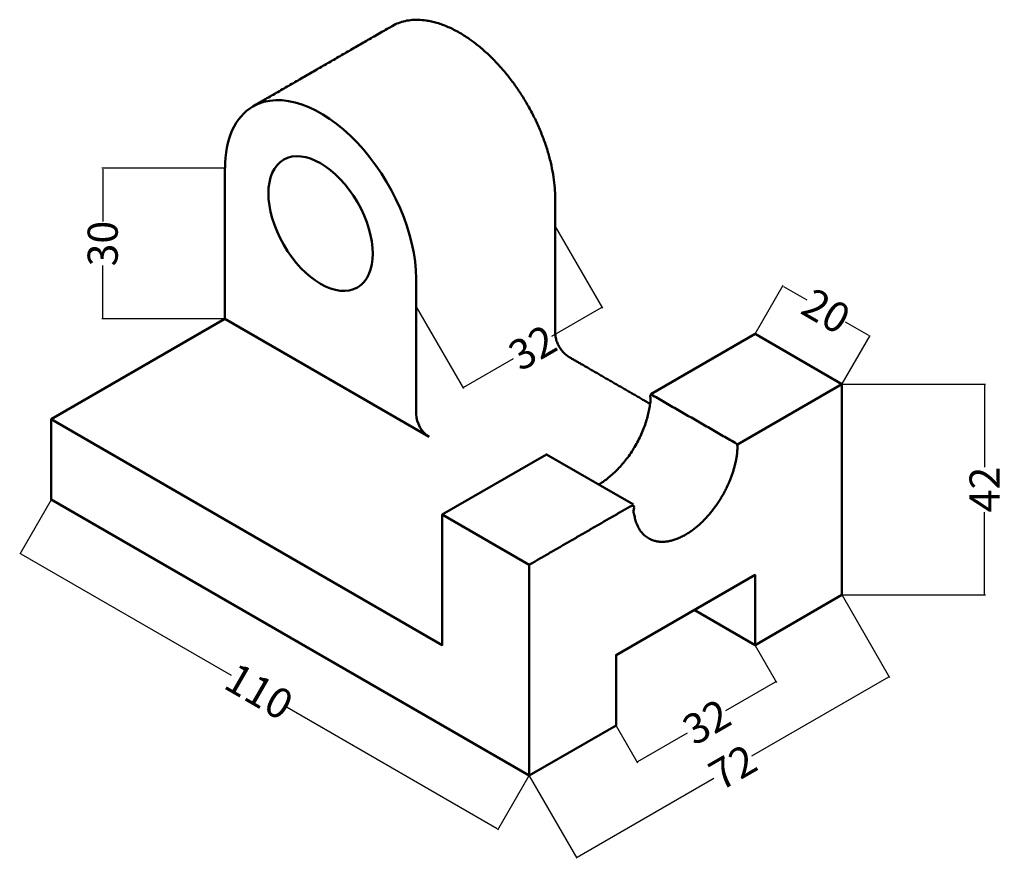
# Model space of a CAD drawing. Units: millimetres. Extents: x -6 to 190, y -9 to 158.
import ezdxf

# ---------------------------------------------------------------- set-up
doc = ezdxf.new("R2010")
doc.units = ezdxf.units.MM
doc.header["$MEASUREMENT"] = 0
doc.layers.add('M-DIMS', color=2, linetype='Continuous', lineweight=25)
doc.layers.add('M-OUTL', color=7, linetype='Continuous', lineweight=50)
doc.styles.get("Standard").update_dxf_attribs({"font": 'arial.ttf'})
doc.dimstyles.get("Standard").update_dxf_attribs({"dimtxt": 6, "dimasz": 0.18, "dimexe": 0.18, "dimexo": 0.0625, "dimgap": 0.09, "dimtad": 0, "dimtoh": 1, "dimdec": 0, "dimzin": 0, "dimdsep": 46, "dimtxsty": 'Standard', "dimcen": 0.09, "dimadec": 0, "dimazin": 0, "dimtfac": 1, "dimtdec": 0, "dimtofl": 0, "dimtmove": 0, "dimatfit": 3, "dimfxl": 1, "dimtolj": 1, "dimtzin": 0, "dimarcsym": 0})

# ---------------------------------------------------------------- blocks, each defined once
blk = doc.blocks.new('*D1')
at = {"layer": 'Defpoints', "color": 0, "transparency": 16777216}
for p in [(157.45, 85.07), (157.45, 43.07), (185.88, 43.07)]:
    blk.add_point(p, dxfattribs=at)
at = {"layer": 'M-DIMS', "color": 0, "lineweight": -2, "transparency": 16777216}
for p, q in [((157.51, 85.07), (186.06, 85.07)), ((185.88, 84.89), (185.88, 68.55)), ((185.88, 43.25), (185.88, 59.59)), ((157.51, 43.07), (186.06, 43.07))]:
    blk.add_line(p, q, dxfattribs=at)
at = {"layer": 'M-DIMS', "color": 0, "transparency": 16777216}
for points in [[(185.85, 84.89), (185.91, 84.89), (185.88, 85.07)], [(185.85, 43.25), (185.91, 43.25), (185.88, 43.07)]]:
    blk.add_solid(points, dxfattribs=at)
at = {"layer": 'M-DIMS', "color": 0, "transparency": 16777216, "insert": (185.88, 64.07), "char_height": 6, "attachment_point": 5, "rotation": 90}
blk.add_mtext('\\A1;42', dxfattribs=at)
blk = doc.blocks.new('*D2')
at = {"layer": 'Defpoints', "color": 0, "transparency": 16777216}
for p in [(-0.17, 62.07), (95.1, 7.07), (88.91, -3.65)]:
    blk.add_point(p, dxfattribs=at)
at = {"layer": 'M-DIMS', "color": 0, "lineweight": -2, "transparency": 16777216}
for p, q in [((-0.2, 62.02), (-6.45, 51.2)), ((-6.2, 51.26), (35.71, 27.07)), ((88.75, -3.56), (46.84, 20.64)), ((95.06, 7.02), (88.82, -3.8))]:
    blk.add_line(p, q, dxfattribs=at)
at = {"layer": 'M-DIMS', "color": 0, "transparency": 16777216}
for points in [[(-6.18, 51.29), (-6.21, 51.24), (-6.36, 51.35)], [(88.77, -3.53), (88.74, -3.58), (88.91, -3.65)]]:
    blk.add_solid(points, dxfattribs=at)
at = {"layer": 'M-DIMS', "color": 0, "transparency": 16777216, "insert": (41.28, 23.85), "char_height": 6, "attachment_point": 5, "rotation": 330}
blk.add_mtext('\\A1;110', dxfattribs=at)
blk = doc.blocks.new('*D3')
at = {"layer": 'Defpoints', "color": 0, "transparency": 16777216}
for p in [(157.45, 43.07), (166.87, 26.75), (95.1, 7.07)]:
    blk.add_point(p, dxfattribs=at)
at = {"layer": 'M-DIMS', "color": 0, "lineweight": -2, "transparency": 16777216}
for p, q in [((157.48, 43.02), (166.96, 26.6)), ((166.71, 26.66), (139.45, 10.92)), ((95.13, 7.02), (104.61, -9.4)), ((104.67, -9.16), (131.94, 6.59))]:
    blk.add_line(p, q, dxfattribs=at)
at = {"layer": 'M-DIMS', "color": 0, "transparency": 16777216}
for points in [[(166.7, 26.69), (166.73, 26.64), (166.87, 26.75)], [(104.66, -9.13), (104.69, -9.18), (104.52, -9.25)]]:
    blk.add_solid(points, dxfattribs=at)
at = {"layer": 'M-DIMS', "color": 0, "transparency": 16777216, "insert": (135.69, 8.75), "char_height": 6, "attachment_point": 5, "rotation": 30}
blk.add_mtext('\\A1;72', dxfattribs=at)
blk = doc.blocks.new('*D4')
at = {"layer": 'Defpoints', "color": 0, "transparency": 16777216}
for p in [(140.13, 33.07), (144.33, 25.79), (112.42, 17.07)]:
    blk.add_point(p, dxfattribs=at)
at = {"layer": 'M-DIMS', "color": 0, "lineweight": -2, "transparency": 16777216}
for p, q in [((140.16, 33.02), (144.42, 25.64)), ((144.17, 25.7), (134.24, 19.97)), ((112.45, 17.02), (116.71, 9.64)), ((116.77, 9.88), (126.7, 15.62))]:
    blk.add_line(p, q, dxfattribs=at)
at = {"layer": 'M-DIMS', "color": 0, "transparency": 16777216}
for points in [[(144.16, 25.73), (144.19, 25.68), (144.33, 25.79)], [(116.76, 9.91), (116.79, 9.86), (116.62, 9.79)]]:
    blk.add_solid(points, dxfattribs=at)
at = {"layer": 'M-DIMS', "color": 0, "transparency": 16777216, "insert": (130.47, 17.79), "char_height": 6, "attachment_point": 5, "rotation": 30}
blk.add_mtext('\\A1;32', dxfattribs=at)
blk = doc.blocks.new('*D5')
at = {"layer": 'Defpoints', "color": 0, "transparency": 16777216}
for p in [(140.13, 95.07), (162.97, 94.64), (157.45, 85.07)]:
    blk.add_point(p, dxfattribs=at)
at = {"layer": 'M-DIMS', "color": 0, "lineweight": -2, "transparency": 16777216}
for p, q in [((140.16, 95.12), (145.74, 104.79)), ((145.81, 104.55), (150.48, 101.85)), ((162.82, 94.73), (158.15, 97.42)), ((157.48, 85.12), (163.06, 94.79))]:
    blk.add_line(p, q, dxfattribs=at)
at = {"layer": 'M-DIMS', "color": 0, "transparency": 16777216}
for points in [[(145.82, 104.57), (145.79, 104.52), (145.65, 104.64)], [(162.83, 94.75), (162.8, 94.7), (162.97, 94.64)]]:
    blk.add_solid(points, dxfattribs=at)
at = {"layer": 'M-DIMS', "color": 0, "transparency": 16777216, "insert": (154.31, 99.64), "char_height": 6, "attachment_point": 5, "rotation": 330}
blk.add_mtext('\\A1;20', dxfattribs=at)
blk = doc.blocks.new('*D6')
at = {"layer": 'Defpoints', "color": 0, "transparency": 16777216}
for p in [(34.47, 128.07), (10.1, 98.07), (34.47, 98.07)]:
    blk.add_point(p, dxfattribs=at)
at = {"layer": 'M-DIMS', "color": 0, "lineweight": -2, "transparency": 16777216}
for p, q in [((34.41, 128.07), (9.92, 128.07)), ((10.1, 127.89), (10.1, 117.45)), ((10.1, 98.25), (10.1, 108.7)), ((34.41, 98.07), (9.92, 98.07))]:
    blk.add_line(p, q, dxfattribs=at)
at = {"layer": 'M-DIMS', "color": 0, "transparency": 16777216}
for points in [[(10.07, 127.89), (10.13, 127.89), (10.1, 128.07)], [(10.07, 98.25), (10.13, 98.25), (10.1, 98.07)]]:
    blk.add_solid(points, dxfattribs=at)
at = {"layer": 'M-DIMS', "color": 0, "transparency": 16777216, "insert": (10.1, 113.07), "char_height": 6, "attachment_point": 5, "rotation": 90}
blk.add_mtext('\\A1;30', dxfattribs=at)
blk = doc.blocks.new('*D7')
at = {"layer": 'Defpoints', "color": 0, "transparency": 16777216}
for p in [(100.29, 116.52), (72.58, 100.52), (109.62, 100.36)]:
    blk.add_point(p, dxfattribs=at)
at = {"layer": 'M-DIMS', "color": 0, "lineweight": -2, "transparency": 16777216}
for p, q in [((100.32, 116.47), (109.71, 100.21)), ((72.61, 100.47), (82, 84.21)), ((109.47, 100.27), (99.54, 94.54)), ((82.07, 84.45), (91.99, 90.19))]:
    blk.add_line(p, q, dxfattribs=at)
at = {"layer": 'M-DIMS', "color": 0, "transparency": 16777216}
for points in [[(109.45, 100.3), (109.48, 100.25), (109.62, 100.36)], [(82.05, 84.48), (82.08, 84.43), (81.91, 84.36)]]:
    blk.add_solid(points, dxfattribs=at)
at = {"layer": 'M-DIMS', "color": 0, "transparency": 16777216, "insert": (95.77, 92.36), "char_height": 6, "attachment_point": 5, "rotation": 30}
blk.add_mtext('\\A1;32', dxfattribs=at)

msp = doc.modelspace()

# ---------------------------------------------------------------- linework, layer by layer
at = {"layer": 'M-OUTL'}
for p, q in [((34.47, 98.07), (34.47, 128.07)), ((72.58, 106.07), (72.58, 79.07)), ((75.18, 74.57), (34.47, 98.07))]:
    msp.add_line(p, q, dxfattribs=at)
for points in [[(34.47, 98.07), (-0.17, 78.07), (-0.17, 62.07), (95.1, 7.07), (112.42, 17.07), (112.42, 31.07), (140.13, 47.07), (140.13, 33.07), (128, 40.07)], [(119.34, 83.07), (140.13, 95.07), (157.45, 85.07), (136.66, 73.07)], [(140.13, 33.07), (157.45, 43.07), (157.45, 85.07)], [(77.77, 59.07), (77.77, 33.07), (-0.17, 78.07)], [(95.1, 7.07), (95.1, 49.07), (77.77, 59.07), (98.56, 71.07), (115.88, 61.07)]]:
    msp.add_lwpolyline(points, dxfattribs=at)
for centre, major_axis, start_param, end_param in [((53.53, 117.07), (13.47, -23.33), 0.785398, 3.141593), ((53.53, 117.07), (13.47, -23.33), 3.141593, 3.926991), ((75.18, 77.57), (-1.84, 3.18), 0.785398, 2.356194)]:
    msp.add_ellipse(centre, major_axis=major_axis, ratio=0.57735, start_param=start_param, end_param=end_param, dxfattribs=at)
msp.add_ellipse((53.53, 117.07), major_axis=(7.35, -12.73), ratio=0.57735, dxfattribs=at)
for points, weights, knots in [([(119.22, 81.14), (111.26, 85.74), (103.29, 90.34), (100.29, 92.07), (100.29, 95.53), (100.29, 108.8), (100.29, 122.07), (100.29, 136.77), (88.53, 149.19), (76.77, 161.6), (67.77, 156.41), (53.91, 148.41), (40.05, 140.41)], [1, 1, 1, 0.866025403784, 1, 1, 1, 0.831469612303, 1, 0.831469612303, 1, 1, 1], [0, 0, 0, 1, 1, 2.047198, 2.047198, 3.047198, 3.047198, 4.225295, 4.225295, 5.403392, 5.403392, 6.403392, 6.403392, 6.403392]), ([(108.95, 65.07), (119.34, 71.07), (119.34, 83.07), (128, 78.07), (136.66, 73.07), (136.66, 66.14), (131.47, 59.68), (126.27, 53.21), (121.08, 53.68), (115.88, 54.14), (115.88, 61.07), (105.49, 55.07), (95.1, 49.07)], [1, 0.707106781187, 1, 1, 1, 0.866025403784, 1, 0.866025403784, 1, 0.866025403784, 1, 1, 1], [0, 0, 0, 1.570796, 1.570796, 2.570796, 2.570796, 3.617994, 3.617994, 4.665191, 4.665191, 5.712389, 5.712389, 6.712389, 6.712389, 6.712389])]:
    msp.add_rational_spline(points, weights, degree=2, knots=knots, dxfattribs=at)

# ---------------------------------------------------------------- dimensions: what is measured, and where the dimension line sits
at = {"layer": 'M-DIMS'}
for p1, p2, distance, picture, middle in [((34.47, 128.07), (34.47, 98.07), -24.38, '*D6', (10.1, 113.07)), ((72.58, 100.52), (100.29, 116.52), -18.66, '*D7', (95.77, 92.36)), ((140.13, 95.07), (157.45, 85.07), 11.05, '*D5', (154.31, 99.64)), ((157.45, 85.07), (157.45, 43.07), 28.43, '*D1', (185.88, 64.07)), ((-0.17, 62.07), (95.1, 7.07), -12.38, '*D2', (41.28, 23.85)), ((95.1, 7.07), (157.45, 43.07), -18.84, '*D3', (135.69, 8.75)), ((112.42, 17.07), (140.13, 33.07), -8.4, '*D4', (130.47, 17.79))]:
    dim = msp.add_aligned_dim(p1=p1, p2=p2, distance=distance, dimstyle='Standard', override={"dimclrd": 0, "dimclre": 0, "dimclrt": 0}, dxfattribs=at)
    dim.commit()
    dim.dimension.update_dxf_attribs({"geometry": picture, "text_midpoint": middle})

doc.saveas('drawing.dxf')
